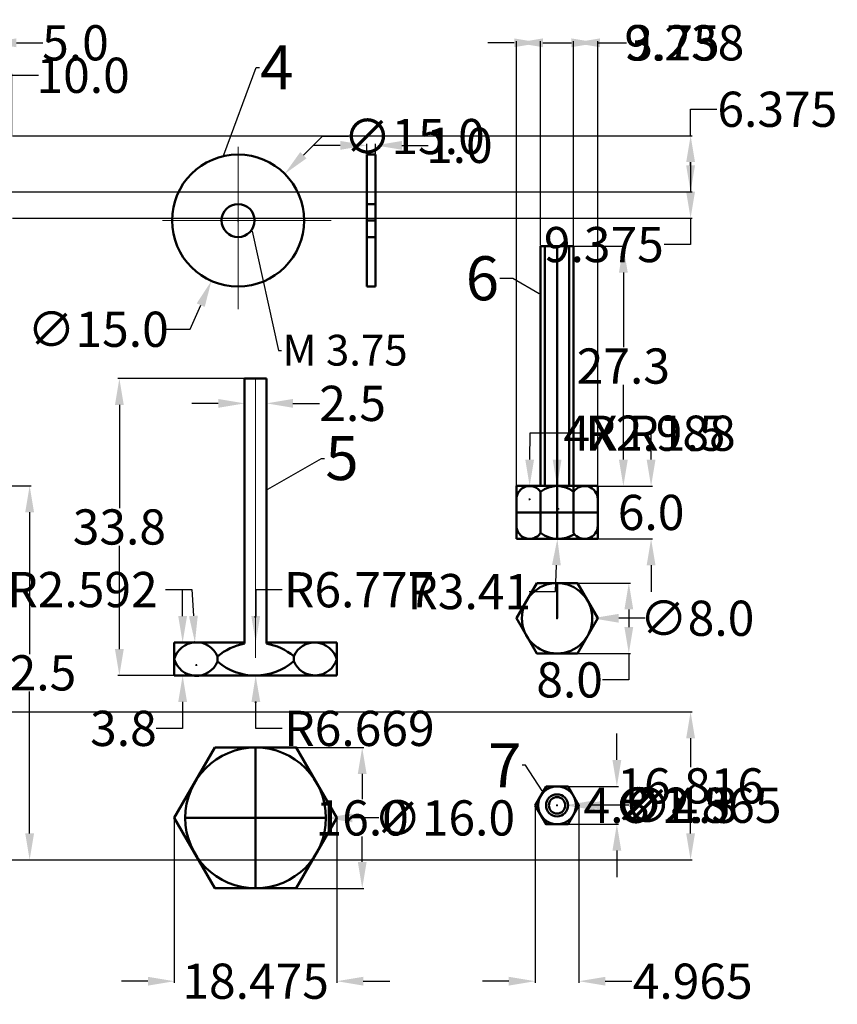
# Model space of a CAD drawing. Units: inches. Extents: x 0 to 231, y -13 to 111.
# Tile 3 of 3: x 138 to 231, y -13 to 98. Entities that reach past the tile are written whole.
import ezdxf
from ezdxf import colors
from ezdxf.entities.mleader import LeaderData, LeaderLine
from ezdxf.math import Vec2, Vec3

# ---------------------------------------------------------------- set-up
doc = ezdxf.new("R2010")
doc.units = ezdxf.units.IN
doc.header["$MEASUREMENT"] = 0
doc.linetypes.add('CENTER', pattern=[50.8, 31.75, -6.35, 6.35, -6.35])
for name, color, linetype, lineweight in [('M-CNTR', 1, 'CENTER', 18), ('M-DIMS', 2, 'Continuous', 25), ('M-OUTL', 7, 'Continuous', 50), ('M-TEXT', 3, 'Continuous', 25)]:
    doc.layers.add(name, color=color, linetype=linetype, lineweight=lineweight)
doc.styles.get("Standard").update_dxf_attribs({"font": 'arial.ttf'})
doc.dimstyles.get("Standard").update_dxf_attribs({"dimtxt": 4, "dimasz": 3, "dimexe": 0.18, "dimexo": 0.0625, "dimgap": 0.09, "dimtad": 0, "dimtih": 1, "dimtoh": 1, "dimdec": 1, "dimzin": 0, "dimdsep": 46, "dimtxsty": 'Standard', "dimcen": 0.09, "dimadec": 0, "dimazin": 0, "dimtfac": 1, "dimtdec": 1, "dimtofl": 0, "dimtmove": 0, "dimatfit": 3, "dimfxl": 1, "dimtolj": 1, "dimtzin": 0, "dimarcsym": 0})

# ---------------------------------------------------------------- blocks, each defined once
blk = doc.blocks.new('*D7')
at = {"layer": 'Defpoints', "color": 0, "transparency": 16777216}
for p in [(136.95, 92.07), (126.95, 85.21), (136.95, 85.21)]:
    blk.add_point(p, dxfattribs=at)
at = {"layer": 'M-DIMS', "color": 0, "lineweight": -2, "transparency": 16777216}
for p, q in [((126.95, 85.27), (126.95, 92.25)), ((129.95, 92.07), (133.95, 92.07)), ((136.95, 85.27), (136.95, 92.25)), ((136.95, 92.07), (139.95, 92.07))]:
    blk.add_line(p, q, dxfattribs=at)
at = {"layer": 'M-DIMS', "color": 0, "transparency": 16777216}
for points in [[(129.95, 92.57), (129.95, 91.57), (126.95, 92.07)], [(133.95, 92.57), (133.95, 91.57), (136.95, 92.07)]]:
    blk.add_solid(points, dxfattribs=at)
at = {"layer": 'M-DIMS', "color": 0, "transparency": 16777216, "insert": (145.04, 92.07), "char_height": 4, "attachment_point": 5}
blk.add_mtext('\\A1;10.0', dxfattribs=at)
blk = doc.blocks.new('*D17')
at = {"layer": 'Defpoints', "color": 0, "transparency": 16777216}
for p in [(120.95, 45.44), (120.95, 2.94), (138.96, 2.94)]:
    blk.add_point(p, dxfattribs=at)
at = {"layer": 'M-DIMS', "color": 0, "lineweight": -2, "transparency": 16777216}
for p, q in [((121.01, 45.44), (139.14, 45.44)), ((138.96, 42.44), (138.96, 26.33)), ((138.96, 5.94), (138.96, 22.06)), ((121.01, 2.94), (139.14, 2.94))]:
    blk.add_line(p, q, dxfattribs=at)
at = {"layer": 'M-DIMS', "color": 0, "transparency": 16777216}
for points in [[(138.46, 42.44), (139.46, 42.44), (138.96, 45.44)], [(138.46, 5.94), (139.46, 5.94), (138.96, 2.94)]]:
    blk.add_solid(points, dxfattribs=at)
at = {"layer": 'M-DIMS', "color": 0, "transparency": 16777216, "insert": (138.96, 24.19), "char_height": 4, "attachment_point": 5}
blk.add_mtext('\\A1;42.5', dxfattribs=at)
blk = doc.blocks.new('*D20')
at = {"layer": 'Defpoints', "color": 0, "transparency": 16777216}
for p in [(165.67, 82.43), (159.62, 68.71)]:
    blk.add_point(p, dxfattribs=at)
at = {"layer": 'M-DIMS', "color": 0, "lineweight": -2, "transparency": 16777216}
for p, q in [((162.56, 75.57), (162.74, 75.57)), ((162.65, 75.48), (162.65, 75.66)), ((157.2, 63.22), (158.41, 65.96)), ((154.2, 63.22), (157.2, 63.22))]:
    blk.add_line(p, q, dxfattribs=at)
at = {"layer": 'M-DIMS', "color": 0, "transparency": 16777216}
blk.add_solid([(157.95, 66.16), (158.86, 65.76), (159.62, 68.71)], dxfattribs=at)
at = {"layer": 'M-DIMS', "color": 0, "transparency": 16777216, "insert": (146.74, 63.22), "char_height": 4, "attachment_point": 5}
blk.add_mtext('\\A1;∅15.0', dxfattribs=at)
blk = doc.blocks.new('*D21')
at = {"layer": 'Defpoints', "color": 0, "transparency": 16777216}
for p in [(178.27, 84.11), (177.27, 83.07), (178.27, 83.07)]:
    blk.add_point(p, dxfattribs=at)
at = {"layer": 'M-DIMS', "color": 0, "lineweight": -2, "transparency": 16777216}
for p, q in [((174.27, 84.11), (171.27, 84.11)), ((177.27, 83.13), (177.27, 84.29)), ((178.27, 83.13), (178.27, 84.29)), ((181.27, 84.11), (184.27, 84.11))]:
    blk.add_line(p, q, dxfattribs=at)
at = {"layer": 'M-DIMS', "color": 0, "transparency": 16777216}
for points in [[(174.27, 84.61), (174.27, 83.61), (177.27, 84.11)], [(181.27, 84.61), (181.27, 83.61), (178.27, 84.11)]]:
    blk.add_solid(points, dxfattribs=at)
at = {"layer": 'M-DIMS', "color": 0, "transparency": 16777216, "insert": (187.8, 84.11), "char_height": 4, "attachment_point": 5}
blk.add_mtext('\\A1;1.0', dxfattribs=at)
blk = doc.blocks.new('*D22')
at = {"layer": 'Defpoints', "color": 0, "transparency": 16777216}
for p in [(164.64, 57.63), (149.16, 23.88), (164.59, 23.88)]:
    blk.add_point(p, dxfattribs=at)
at = {"layer": 'M-DIMS', "color": 0, "lineweight": -2, "transparency": 16777216}
for p, q in [((164.58, 57.63), (148.98, 57.63)), ((149.16, 54.63), (149.16, 42.89)), ((149.16, 26.88), (149.16, 38.62)), ((164.53, 23.88), (148.98, 23.88))]:
    blk.add_line(p, q, dxfattribs=at)
at = {"layer": 'M-DIMS', "color": 0, "transparency": 16777216}
for points in [[(148.66, 54.63), (149.66, 54.63), (149.16, 57.63)], [(148.66, 26.88), (149.66, 26.88), (149.16, 23.88)]]:
    blk.add_solid(points, dxfattribs=at)
at = {"layer": 'M-DIMS', "color": 0, "transparency": 16777216, "insert": (149.16, 40.76), "char_height": 4, "attachment_point": 5}
blk.add_mtext('\\A1;33.8', dxfattribs=at)
blk = doc.blocks.new('*D23')
at = {"layer": 'Defpoints', "color": 0, "transparency": 16777216}
for p in [(155.41, 27.63), (155.41, 23.88), (156.35, 23.88)]:
    blk.add_point(p, dxfattribs=at)
at = {"layer": 'M-DIMS', "color": 0, "lineweight": -2, "transparency": 16777216}
for p, q in [((156.35, 30.63), (156.35, 33.63)), ((155.47, 27.63), (156.53, 27.63)), ((155.47, 23.88), (156.53, 23.88)), ((156.35, 20.88), (156.35, 17.88)), ((156.35, 17.88), (153.35, 17.88))]:
    blk.add_line(p, q, dxfattribs=at)
at = {"layer": 'M-DIMS', "color": 0, "transparency": 16777216}
for points in [[(155.85, 30.63), (156.85, 30.63), (156.35, 27.63)], [(155.85, 20.88), (156.85, 20.88), (156.35, 23.88)]]:
    blk.add_solid(points, dxfattribs=at)
at = {"layer": 'M-DIMS', "color": 0, "transparency": 16777216, "insert": (149.62, 17.88), "char_height": 4, "attachment_point": 5}
blk.add_mtext('\\A1;3.8', dxfattribs=at)
blk = doc.blocks.new('*D24')
at = {"layer": 'Defpoints', "color": 0, "transparency": 16777216}
for p in [(164.64, 15.71), (164.64, -0.29), (176.76, -0.29)]:
    blk.add_point(p, dxfattribs=at)
at = {"layer": 'M-DIMS', "color": 0, "lineweight": -2, "transparency": 16777216}
for p, q in [((164.71, 15.71), (176.94, 15.71)), ((176.76, 12.71), (176.76, 9.84)), ((176.76, 2.71), (176.76, 5.58)), ((164.71, -0.29), (176.94, -0.29))]:
    blk.add_line(p, q, dxfattribs=at)
at = {"layer": 'M-DIMS', "color": 0, "transparency": 16777216}
for points in [[(176.26, 12.71), (177.26, 12.71), (176.76, 15.71)], [(176.26, 2.71), (177.26, 2.71), (176.76, -0.29)]]:
    blk.add_solid(points, dxfattribs=at)
at = {"layer": 'M-DIMS', "color": 0, "transparency": 16777216, "insert": (176.76, 7.71), "char_height": 4, "attachment_point": 5}
blk.add_mtext('\\A1;16.0', dxfattribs=at)
blk = doc.blocks.new('*D25')
at = {"layer": 'Defpoints', "color": 0, "transparency": 16777216}
for p in [(163.39, 53.99), (165.89, 54.8), (165.89, 54.36)]:
    blk.add_point(p, dxfattribs=at)
at = {"layer": 'M-DIMS', "color": 0, "lineweight": -2, "transparency": 16777216}
for p, q in [((163.39, 54.05), (163.39, 54.98)), ((165.89, 54.42), (165.89, 54.98)), ((160.39, 54.8), (157.39, 54.8)), ((168.89, 54.8), (171.89, 54.8))]:
    blk.add_line(p, q, dxfattribs=at)
at = {"layer": 'M-DIMS', "color": 0, "transparency": 16777216}
for points in [[(160.39, 55.3), (160.39, 54.3), (163.39, 54.8)], [(168.89, 55.3), (168.89, 54.3), (165.89, 54.8)]]:
    blk.add_solid(points, dxfattribs=at)
at = {"layer": 'M-DIMS', "color": 0, "transparency": 16777216, "insert": (175.67, 54.8), "char_height": 4, "attachment_point": 5}
blk.add_mtext('\\A1;2.5', dxfattribs=at)
blk = doc.blocks.new('*D26')
at = {"layer": 'Defpoints', "color": 0, "transparency": 16777216}
for p in [(203.53, 45.41), (203.53, 39.41), (209.59, 39.41)]:
    blk.add_point(p, dxfattribs=at)
at = {"layer": 'M-DIMS', "color": 0, "lineweight": -2, "transparency": 16777216}
for p, q in [((209.59, 48.41), (209.59, 51.41)), ((203.59, 45.41), (209.77, 45.41)), ((203.59, 39.41), (209.77, 39.41)), ((209.59, 36.41), (209.59, 33.41))]:
    blk.add_line(p, q, dxfattribs=at)
at = {"layer": 'M-DIMS', "color": 0, "transparency": 16777216}
for points in [[(209.09, 48.41), (210.09, 48.41), (209.59, 45.41)], [(209.09, 36.41), (210.09, 36.41), (209.59, 39.41)]]:
    blk.add_solid(points, dxfattribs=at)
at = {"layer": 'M-DIMS', "color": 0, "transparency": 16777216, "insert": (209.59, 42.41), "char_height": 4, "attachment_point": 5}
blk.add_mtext('\\A1;6.0', dxfattribs=at)
blk = doc.blocks.new('*D27')
at = {"layer": 'Defpoints', "color": 0, "transparency": 16777216}
for p in [(198.91, 72.66), (198.91, 45.41), (206.44, 45.41)]:
    blk.add_point(p, dxfattribs=at)
at = {"layer": 'M-DIMS', "color": 0, "lineweight": -2, "transparency": 16777216}
for p, q in [((198.97, 72.66), (206.62, 72.66)), ((206.44, 69.66), (206.44, 61.17)), ((206.44, 48.41), (206.44, 56.91)), ((198.97, 45.41), (206.62, 45.41))]:
    blk.add_line(p, q, dxfattribs=at)
at = {"layer": 'M-DIMS', "color": 0, "transparency": 16777216}
for points in [[(205.94, 69.66), (206.94, 69.66), (206.44, 72.66)], [(205.94, 48.41), (206.94, 48.41), (206.44, 45.41)]]:
    blk.add_solid(points, dxfattribs=at)
at = {"layer": 'M-DIMS', "color": 0, "transparency": 16777216, "insert": (206.44, 59.04), "char_height": 4, "attachment_point": 5}
blk.add_mtext('\\A1;27.3', dxfattribs=at)
blk = doc.blocks.new('*D28')
at = {"layer": 'Defpoints', "color": 0, "transparency": 16777216}
for p in [(198.91, 34.39), (198.91, 26.39), (207.06, 26.39)]:
    blk.add_point(p, dxfattribs=at)
at = {"layer": 'M-DIMS', "color": 0, "lineweight": -2, "transparency": 16777216}
for p, q in [((198.97, 34.39), (207.24, 34.39)), ((207.06, 31.39), (207.06, 29.39)), ((198.97, 26.39), (207.24, 26.39)), ((207.06, 26.39), (207.06, 23.39)), ((207.06, 23.39), (204.06, 23.39))]:
    blk.add_line(p, q, dxfattribs=at)
at = {"layer": 'M-DIMS', "color": 0, "transparency": 16777216}
for points in [[(206.56, 31.39), (207.56, 31.39), (207.06, 34.39)], [(206.56, 29.39), (207.56, 29.39), (207.06, 26.39)]]:
    blk.add_solid(points, dxfattribs=at)
at = {"layer": 'M-DIMS', "color": 0, "transparency": 16777216, "insert": (200.33, 23.39), "char_height": 4, "attachment_point": 5}
blk.add_mtext('\\A1;8.0', dxfattribs=at)
blk = doc.blocks.new('*D29')
at = {"layer": 'Defpoints', "color": 0, "transparency": 16777216}
for p in [(198.91, 11.29), (198.91, 6.99), (205.7, 6.99)]:
    blk.add_point(p, dxfattribs=at)
at = {"layer": 'M-DIMS', "color": 0, "lineweight": -2, "transparency": 16777216}
for p, q in [((205.7, 14.29), (205.7, 17.29)), ((198.97, 11.29), (205.88, 11.29)), ((198.97, 6.99), (205.88, 6.99)), ((205.7, 3.99), (205.7, 0.99))]:
    blk.add_line(p, q, dxfattribs=at)
at = {"layer": 'M-DIMS', "color": 0, "transparency": 16777216}
for points in [[(205.2, 14.29), (206.2, 14.29), (205.7, 11.29)], [(205.2, 3.99), (206.2, 3.99), (205.7, 6.99)]]:
    blk.add_solid(points, dxfattribs=at)
at = {"layer": 'M-DIMS', "color": 0, "transparency": 16777216, "insert": (205.7, 9.14), "char_height": 4, "attachment_point": 5}
blk.add_mtext('\\A1;4.3', dxfattribs=at)
blk = doc.blocks.new('*D34')
at = {"layer": 'Defpoints', "color": 0, "transparency": 16777216}
for p in [(134.45, 95.76), (129.45, 85.21), (134.45, 85.21)]:
    blk.add_point(p, dxfattribs=at)
at = {"layer": 'M-DIMS', "color": 0, "lineweight": -2, "transparency": 16777216}
for p, q in [((126.45, 95.76), (123.45, 95.76)), ((129.45, 85.27), (129.45, 95.94)), ((134.45, 85.27), (134.45, 95.94)), ((137.45, 95.76), (140.45, 95.76))]:
    blk.add_line(p, q, dxfattribs=at)
at = {"layer": 'M-DIMS', "color": 0, "transparency": 16777216}
for points in [[(126.45, 96.26), (126.45, 95.26), (129.45, 95.76)], [(137.45, 96.26), (137.45, 95.26), (134.45, 95.76)]]:
    blk.add_solid(points, dxfattribs=at)
at = {"layer": 'M-DIMS', "color": 0, "transparency": 16777216, "insert": (144.17, 95.76), "char_height": 4, "attachment_point": 5}
blk.add_mtext('\\A1;5.0', dxfattribs=at)
blk = doc.blocks.new('*D35')
at = {"layer": 'Defpoints', "color": 0, "transparency": 16777216}
for p in [(136.95, 85.21), (214.08, 85.21), (131.95, 78.84)]:
    blk.add_point(p, dxfattribs=at)
at = {"layer": 'M-DIMS', "color": 0, "lineweight": -2, "transparency": 16777216}
for p, q in [((214.08, 85.21), (214.08, 88.21)), ((214.08, 88.21), (217.08, 88.21)), ((137.01, 85.21), (214.26, 85.21)), ((214.08, 81.84), (214.08, 82.21)), ((132.01, 78.84), (214.26, 78.84))]:
    blk.add_line(p, q, dxfattribs=at)
at = {"layer": 'M-DIMS', "color": 0, "transparency": 16777216}
for points in [[(213.58, 82.21), (214.58, 82.21), (214.08, 85.21)], [(213.58, 81.84), (214.58, 81.84), (214.08, 78.84)]]:
    blk.add_solid(points, dxfattribs=at)
at = {"layer": 'M-DIMS', "color": 0, "transparency": 16777216, "insert": (223.94, 88.21), "char_height": 4, "attachment_point": 5}
blk.add_mtext('\\A1;6.375', dxfattribs=at)
blk = doc.blocks.new('*D36')
at = {"layer": 'Defpoints', "color": 0, "transparency": 16777216}
for p in [(136.95, 85.21), (136.95, 75.84), (214.08, 75.84)]:
    blk.add_point(p, dxfattribs=at)
at = {"layer": 'M-DIMS', "color": 0, "lineweight": -2, "transparency": 16777216}
for p, q in [((137.01, 85.21), (214.26, 85.21)), ((214.08, 82.21), (214.08, 78.84)), ((137.01, 75.84), (214.26, 75.84)), ((214.08, 75.84), (214.08, 72.84)), ((214.08, 72.84), (211.08, 72.84))]:
    blk.add_line(p, q, dxfattribs=at)
at = {"layer": 'M-DIMS', "color": 0, "transparency": 16777216}
for points in [[(213.58, 82.21), (214.58, 82.21), (214.08, 85.21)], [(213.58, 78.84), (214.58, 78.84), (214.08, 75.84)]]:
    blk.add_solid(points, dxfattribs=at)
at = {"layer": 'M-DIMS', "color": 0, "transparency": 16777216, "insert": (204.22, 72.84), "char_height": 4, "attachment_point": 5}
blk.add_mtext('\\A1;9.375', dxfattribs=at)
blk = doc.blocks.new('*D45')
at = {"layer": 'Defpoints', "color": 0, "transparency": 16777216}
for p in [(119.7, 19.76), (120.95, 2.94), (214.08, 2.94)]:
    blk.add_point(p, dxfattribs=at)
at = {"layer": 'M-DIMS', "color": 0, "lineweight": -2, "transparency": 16777216}
for p, q in [((119.76, 19.76), (214.26, 19.76)), ((214.08, 16.76), (214.08, 13.48)), ((214.08, 5.94), (214.08, 9.22)), ((121.01, 2.94), (214.26, 2.94))]:
    blk.add_line(p, q, dxfattribs=at)
at = {"layer": 'M-DIMS', "color": 0, "transparency": 16777216}
for points in [[(213.58, 16.76), (214.58, 16.76), (214.08, 19.76)], [(213.58, 5.94), (214.58, 5.94), (214.08, 2.94)]]:
    blk.add_solid(points, dxfattribs=at)
at = {"layer": 'M-DIMS', "color": 0, "transparency": 16777216, "insert": (214.08, 11.35), "char_height": 4, "attachment_point": 5}
blk.add_mtext('\\A1;16.816', dxfattribs=at)
blk = doc.blocks.new('*D47')
at = {"layer": 'Defpoints', "color": 0, "transparency": 16777216}
for p in [(155.405372, 7.711161), (173.88058, 7.711161), (173.88058, -10.838839)]:
    blk.add_point(p, dxfattribs=at)
at = {"layer": 'M-DIMS', "color": 0, "lineweight": -2, "transparency": 16777216}
for p, q in [((155.405372, 7.648661), (155.405372, -11.018839)), ((173.88058, 7.648661), (173.88058, -11.018839)), ((152.405372, -10.838839), (149.405372, -10.838839)), ((176.88058, -10.838839), (179.88058, -10.838839))]:
    blk.add_line(p, q, dxfattribs=at)
at = {"layer": 'M-DIMS', "color": 0, "transparency": 16777216}
for points in [[(152.405372, -10.338839), (152.405372, -11.338839), (155.405372, -10.838839)], [(176.88058, -10.338839), (176.88058, -11.338839), (173.88058, -10.838839)]]:
    blk.add_solid(points, dxfattribs=at)
at = {"layer": 'M-DIMS', "color": 0, "transparency": 16777216, "insert": (164.642976, -10.838839), "char_height": 4, "attachment_point": 5}
blk.add_mtext('\\A1;18.475', dxfattribs=at)
blk = doc.blocks.new('*D48')
at = {"layer": 'Defpoints', "color": 0, "transparency": 16777216}
for p in [(203.53, 95.76), (194.29, 45.41), (203.53, 45.41)]:
    blk.add_point(p, dxfattribs=at)
at = {"layer": 'M-DIMS', "color": 0, "lineweight": -2, "transparency": 16777216}
for p, q in [((194.29, 45.48), (194.29, 95.94)), ((197.29, 95.76), (200.53, 95.76)), ((203.53, 45.48), (203.53, 95.94)), ((203.53, 95.76), (206.53, 95.76))]:
    blk.add_line(p, q, dxfattribs=at)
at = {"layer": 'M-DIMS', "color": 0, "transparency": 16777216}
for points in [[(197.29, 96.26), (197.29, 95.26), (194.29, 95.76)], [(200.53, 96.26), (200.53, 95.26), (203.53, 95.76)]]:
    blk.add_solid(points, dxfattribs=at)
at = {"layer": 'M-DIMS', "color": 0, "transparency": 16777216, "insert": (213.37, 95.76), "char_height": 4, "attachment_point": 5}
blk.add_mtext('\\A1;9.238', dxfattribs=at)
blk = doc.blocks.new('*D49')
at = {"layer": 'Defpoints', "color": 0, "transparency": 16777216}
for p in [(200.78, 95.76), (197.03, 72.66), (200.78, 72.66)]:
    blk.add_point(p, dxfattribs=at)
at = {"layer": 'M-DIMS', "color": 0, "lineweight": -2, "transparency": 16777216}
for p, q in [((194.03, 95.76), (191.03, 95.76)), ((197.03, 72.73), (197.03, 95.94)), ((200.78, 72.73), (200.78, 95.94)), ((203.78, 95.76), (206.78, 95.76))]:
    blk.add_line(p, q, dxfattribs=at)
at = {"layer": 'M-DIMS', "color": 0, "transparency": 16777216}
for points in [[(194.03, 96.26), (194.03, 95.26), (197.03, 95.76)], [(203.78, 96.26), (203.78, 95.26), (200.78, 95.76)]]:
    blk.add_solid(points, dxfattribs=at)
at = {"layer": 'M-DIMS', "color": 0, "transparency": 16777216, "insert": (212.08, 95.76), "char_height": 4, "attachment_point": 5}
blk.add_mtext('\\A1;3.75', dxfattribs=at)
blk = doc.blocks.new('*D50')
at = {"layer": 'Defpoints', "color": 0, "transparency": 16777216}
for p in [(196.42, 9.14), (201.39, 9.14), (201.39, -10.84)]:
    blk.add_point(p, dxfattribs=at)
at = {"layer": 'M-DIMS', "color": 0, "lineweight": -2, "transparency": 16777216}
for p, q in [((196.42, 9.08), (196.42, -11.02)), ((201.39, 9.08), (201.39, -11.02)), ((193.42, -10.84), (190.42, -10.84)), ((204.39, -10.84), (207.39, -10.84))]:
    blk.add_line(p, q, dxfattribs=at)
at = {"layer": 'M-DIMS', "color": 0, "transparency": 16777216}
for points in [[(193.42, -10.34), (193.42, -11.34), (196.42, -10.84)], [(204.39, -10.34), (204.39, -11.34), (201.39, -10.84)]]:
    blk.add_solid(points, dxfattribs=at)
at = {"layer": 'M-DIMS', "color": 0, "transparency": 16777216, "insert": (214.32, -10.84), "char_height": 4, "attachment_point": 5}
blk.add_mtext('\\A1;4.965', dxfattribs=at)
blk = doc.blocks.new('*D53')
at = {"layer": 'Defpoints', "color": 0, "transparency": 16777216}
for p in [(167.95, 80.87), (157.34, 70.27)]:
    blk.add_point(p, dxfattribs=at)
at = {"layer": 'M-DIMS', "color": 0, "lineweight": -2, "transparency": 16777216}
for p, q in [((172.19, 85.11), (170.07, 82.99)), ((175.19, 85.11), (172.19, 85.11)), ((162.56, 75.57), (162.74, 75.57)), ((162.65, 75.48), (162.65, 75.66))]:
    blk.add_line(p, q, dxfattribs=at)
at = {"layer": 'M-DIMS', "color": 0, "transparency": 16777216}
blk.add_solid([(169.72, 83.35), (170.43, 82.64), (167.95, 80.87)], dxfattribs=at)
at = {"layer": 'M-DIMS', "color": 0, "transparency": 16777216, "insert": (182.65, 85.11), "char_height": 4, "attachment_point": 5}
blk.add_mtext('\\A1;∅15.0', dxfattribs=at)
blk = doc.blocks.new('*D55')
at = {"layer": 'Defpoints', "color": 0, "transparency": 16777216}
for p in [(156.64, 7.71), (172.64, 7.71)]:
    blk.add_point(p, dxfattribs=at)
at = {"layer": 'M-DIMS', "color": 0, "lineweight": -2, "transparency": 16777216}
for p, q in [((164.55, 7.71), (164.73, 7.71)), ((164.64, 7.62), (164.64, 7.8)), ((178.64, 7.71), (175.64, 7.71))]:
    blk.add_line(p, q, dxfattribs=at)
at = {"layer": 'M-DIMS', "color": 0, "transparency": 16777216}
blk.add_solid([(175.64, 8.21), (175.64, 7.21), (172.64, 7.71)], dxfattribs=at)
at = {"layer": 'M-DIMS', "color": 0, "transparency": 16777216, "insert": (186.1, 7.71), "char_height": 4, "attachment_point": 5}
blk.add_mtext('\\A1;∅16.0', dxfattribs=at)
blk = doc.blocks.new('*D56')
at = {"layer": 'Defpoints', "color": 0, "transparency": 16777216}
for p in [(164.66, 27.63), (164.66, 20.86)]:
    blk.add_point(p, dxfattribs=at)
at = {"layer": 'M-DIMS', "color": 0, "lineweight": -2, "transparency": 16777216}
for p, q in [((167.66, 33.63), (164.66, 33.63)), ((164.66, 33.63), (164.66, 30.63)), ((164.57, 20.86), (164.75, 20.86)), ((164.66, 20.77), (164.66, 20.95))]:
    blk.add_line(p, q, dxfattribs=at)
at = {"layer": 'M-DIMS', "color": 0, "transparency": 16777216}
blk.add_solid([(164.16, 30.63), (165.16, 30.63), (164.66, 27.63)], dxfattribs=at)
at = {"layer": 'M-DIMS', "color": 0, "transparency": 16777216, "insert": (176.41, 33.63), "char_height": 4, "attachment_point": 5}
blk.add_mtext('\\A1;R6.777', dxfattribs=at)
blk = doc.blocks.new('*D57')
at = {"layer": 'Defpoints', "color": 0, "transparency": 16777216}
for p in [(164.62, 30.55), (164.65, 23.88)]:
    blk.add_point(p, dxfattribs=at)
at = {"layer": 'M-DIMS', "color": 0, "lineweight": -2, "transparency": 16777216}
for p, q in [((164.53, 30.55), (164.71, 30.55)), ((164.62, 30.46), (164.62, 30.64)), ((164.68, 17.88), (164.67, 20.88)), ((167.68, 17.88), (164.68, 17.88))]:
    blk.add_line(p, q, dxfattribs=at)
at = {"layer": 'M-DIMS', "color": 0, "transparency": 16777216}
blk.add_solid([(165.17, 20.89), (164.17, 20.88), (164.65, 23.88)], dxfattribs=at)
at = {"layer": 'M-DIMS', "color": 0, "transparency": 16777216, "insert": (176.44, 17.88), "char_height": 4, "attachment_point": 5}
blk.add_mtext('\\A1;R6.669', dxfattribs=at)
blk = doc.blocks.new('*D58')
at = {"layer": 'Defpoints', "color": 0, "transparency": 16777216}
for p in [(157.75, 27.66), (157.91, 25.07)]:
    blk.add_point(p, dxfattribs=at)
at = {"layer": 'M-DIMS', "color": 0, "lineweight": -2, "transparency": 16777216}
for p, q in [((154.39, 33.65), (157.39, 33.65)), ((157.39, 33.65), (157.57, 30.65)), ((157.82, 25.07), (158, 25.07)), ((157.91, 24.98), (157.91, 25.16))]:
    blk.add_line(p, q, dxfattribs=at)
at = {"layer": 'M-DIMS', "color": 0, "transparency": 16777216}
blk.add_solid([(158.07, 30.68), (157.07, 30.62), (157.75, 27.66)], dxfattribs=at)
at = {"layer": 'M-DIMS', "color": 0, "transparency": 16777216, "insert": (141.28, 33.65), "char_height": 4, "attachment_point": 5}
blk.add_mtext('\\A1;4X R2.592', dxfattribs=at)
blk = doc.blocks.new('*D59')
at = {"layer": 'Defpoints', "color": 0, "transparency": 16777216}
for p in [(195.79, 45.41), (195.79, 43.91)]:
    blk.add_point(p, dxfattribs=at)
at = {"layer": 'M-DIMS', "color": 0, "lineweight": -2, "transparency": 16777216}
for p, q in [((195.8, 51.41), (195.79, 48.41)), ((198.8, 51.41), (195.8, 51.41)), ((195.7, 43.91), (195.88, 43.91)), ((195.79, 43.82), (195.79, 44))]:
    blk.add_line(p, q, dxfattribs=at)
at = {"layer": 'M-DIMS', "color": 0, "transparency": 16777216}
blk.add_solid([(195.29, 48.42), (196.29, 48.41), (195.79, 45.41)], dxfattribs=at)
at = {"layer": 'M-DIMS', "color": 0, "transparency": 16777216, "insert": (208.84, 51.41), "char_height": 4, "attachment_point": 5}
blk.add_mtext('\\A1;4X R1.5', dxfattribs=at)
blk = doc.blocks.new('*D60')
at = {"layer": 'Defpoints', "color": 0, "transparency": 16777216}
for p in [(199.05, 42.82), (198.94, 39.41)]:
    blk.add_point(p, dxfattribs=at)
at = {"layer": 'M-DIMS', "color": 0, "lineweight": -2, "transparency": 16777216}
for p, q in [((198.96, 42.82), (199.14, 42.82)), ((199.05, 42.73), (199.05, 42.91)), ((198.73, 33.42), (198.83, 36.42)), ((195.73, 33.42), (198.73, 33.42))]:
    blk.add_line(p, q, dxfattribs=at)
at = {"layer": 'M-DIMS', "color": 0, "transparency": 16777216}
blk.add_solid([(198.33, 36.43), (199.33, 36.4), (198.94, 39.41)], dxfattribs=at)
at = {"layer": 'M-DIMS', "color": 0, "transparency": 16777216, "insert": (188.92, 33.42), "char_height": 4, "attachment_point": 5}
blk.add_mtext('\\A1;R3.41', dxfattribs=at)
blk = doc.blocks.new('*D61')
at = {"layer": 'Defpoints', "color": 0, "transparency": 16777216}
for p in [(198.91, 45.41), (198.91, 42.43)]:
    blk.add_point(p, dxfattribs=at)
at = {"layer": 'M-DIMS', "color": 0, "lineweight": -2, "transparency": 16777216}
for p, q in [((201.91, 51.41), (198.91, 51.41)), ((198.91, 51.41), (198.91, 48.41)), ((198.91, 42.34), (198.91, 42.52)), ((198.82, 42.43), (199, 42.43))]:
    blk.add_line(p, q, dxfattribs=at)
at = {"layer": 'M-DIMS', "color": 0, "transparency": 16777216}
blk.add_solid([(198.41, 48.41), (199.41, 48.41), (198.91, 45.41)], dxfattribs=at)
at = {"layer": 'M-DIMS', "color": 0, "transparency": 16777216, "insert": (210.66, 51.41), "char_height": 4, "attachment_point": 5}
blk.add_mtext('\\A1;R2.988', dxfattribs=at)
blk = doc.blocks.new('*D62')
at = {"layer": 'Defpoints', "color": 0, "transparency": 16777216}
for p in [(194.91, 30.39), (202.91, 30.39)]:
    blk.add_point(p, dxfattribs=at)
at = {"layer": 'M-DIMS', "color": 0, "lineweight": -2, "transparency": 16777216}
for p, q in [((198.82, 30.39), (199, 30.39)), ((198.91, 30.3), (198.91, 30.48)), ((208.91, 30.39), (205.91, 30.39))]:
    blk.add_line(p, q, dxfattribs=at)
at = {"layer": 'M-DIMS', "color": 0, "transparency": 16777216}
blk.add_solid([(205.91, 30.89), (205.91, 29.89), (202.91, 30.39)], dxfattribs=at)
at = {"layer": 'M-DIMS', "color": 0, "transparency": 16777216, "insert": (214.81, 30.39), "char_height": 4, "attachment_point": 5}
blk.add_mtext('\\A1;∅8.0', dxfattribs=at)
blk = doc.blocks.new('*D63')
at = {"layer": 'Defpoints', "color": 0, "transparency": 16777216}
for p in [(196.76, 9.14), (201.06, 9.14)]:
    blk.add_point(p, dxfattribs=at)
at = {"layer": 'M-DIMS', "color": 0, "lineweight": -2, "transparency": 16777216}
for p, q in [((198.82, 9.14), (199, 9.14)), ((198.91, 9.05), (198.91, 9.23)), ((207.06, 9.14), (204.06, 9.14))]:
    blk.add_line(p, q, dxfattribs=at)
at = {"layer": 'M-DIMS', "color": 0, "transparency": 16777216}
blk.add_solid([(204.06, 9.64), (204.06, 8.64), (201.06, 9.14)], dxfattribs=at)
at = {"layer": 'M-DIMS', "color": 0, "transparency": 16777216, "insert": (212.96, 9.14), "char_height": 4, "attachment_point": 5}
blk.add_mtext('\\A1;∅4.3', dxfattribs=at)
blk = doc.blocks.new('*D64')
at = {"layer": 'Defpoints', "color": 0, "transparency": 16777216}
for p in [(197.66, 9.14), (200.16, 9.14)]:
    blk.add_point(p, dxfattribs=at)
at = {"layer": 'M-DIMS', "color": 0, "lineweight": -2, "transparency": 16777216}
for p, q in [((198.82, 9.14), (199, 9.14)), ((198.91, 9.05), (198.91, 9.23)), ((206.16, 9.15), (203.16, 9.14))]:
    blk.add_line(p, q, dxfattribs=at)
at = {"layer": 'M-DIMS', "color": 0, "transparency": 16777216}
blk.add_solid([(203.16, 9.64), (203.16, 8.64), (200.16, 9.14)], dxfattribs=at)
at = {"layer": 'M-DIMS', "color": 0, "transparency": 16777216, "insert": (212.08, 9.15), "char_height": 4, "attachment_point": 5}
blk.add_mtext('\\A1;∅2.5', dxfattribs=at)
blk = doc.blocks.new('*D65')
at = {"layer": 'Defpoints', "color": 0, "transparency": 16777216}
for p in [(197.97, 9.14), (199.84, 9.14)]:
    blk.add_point(p, dxfattribs=at)
at = {"layer": 'M-DIMS', "color": 0, "lineweight": -2, "transparency": 16777216}
for p, q in [((198.82, 9.14), (199, 9.14)), ((198.91, 9.05), (198.91, 9.23)), ((205.84, 9.15), (202.84, 9.15))]:
    blk.add_line(p, q, dxfattribs=at)
at = {"layer": 'M-DIMS', "color": 0, "transparency": 16777216}
blk.add_solid([(202.84, 9.65), (202.84, 8.65), (199.84, 9.14)], dxfattribs=at)
at = {"layer": 'M-DIMS', "color": 0, "transparency": 16777216, "insert": (214.87, 9.15), "char_height": 4, "attachment_point": 5}
blk.add_mtext('\\A1;∅1.865', dxfattribs=at)

msp = doc.modelspace()

# ---------------------------------------------------------------- linework, layer by layer
at = {"layer": 'M-CNTR'}
for p, q in [((162.6462, 65.5196), (162.6462, 83.9575)), ((154.0559, 75.5682), (173.2454, 75.5682)), ((164.643, 57.6328), (164.643, 20.2824))]:
    msp.add_line(p, q, dxfattribs=at)
at = {"layer": 'M-OUTL'}
for p, q in [((177.2674, 83.0682), (178.2674, 83.0682)), ((177.2674, 83.0682), (177.2674, 68.0682)), ((178.2674, 83.0682), (178.2674, 68.0682)), ((177.2674, 77.4432), (178.2674, 77.4432)), ((177.2674, 75.5682), (178.2674, 75.5682)), ((177.2674, 73.6932), (178.2674, 73.6932)), ((197.0319, 72.6646), (200.7819, 72.6646)), ((197.0319, 45.4146), (197.0319, 72.6646)), ((197.5319, 45.4146), (197.5319, 72.6646)), ((198.9069, 39.4146), (198.9069, 72.6646)), ((200.2819, 45.4146), (200.2819, 72.6646)), ((200.7819, 40.0761), (200.7819, 72.6646)), ((177.2674, 68.0682), (178.2674, 68.0682)), ((163.393, 57.6328), (165.893, 57.6328)), ((163.393, 57.6328), (163.393, 27.5141)), ((165.893, 57.6328), (165.893, 27.5189)), ((194.2881, 39.4146), (194.2881, 45.4146)), ((194.2881, 45.4146), (203.5257, 45.4146)), ((197.0319, 40.0761), (197.0319, 44.753)), ((203.5257, 39.4146), (203.5257, 45.4146)), ((194.2881, 42.4146), (203.5257, 42.4146)), ((194.2881, 39.4146), (203.5257, 39.4146)), ((198.9069, 30.3883), (198.9069, 34.3883)), ((155.4054, 23.8828), (155.4054, 27.6328)), ((155.4054, 27.6328), (163.393, 27.6328)), ((164.643, 27.6328), (164.6687, 27.6328)), ((165.893, 27.6328), (173.8806, 27.6328)), ((173.8806, 23.8828), (173.8806, 27.6328)), ((160.3054, 25.4635), (160.3054, 26.0521)), ((168.9806, 25.5088), (168.9806, 26.0735)), ((155.4054, 23.8828), (173.8806, 23.8828)), ((163.393, 23.9959), (163.393, 23.8828)), ((165.893, 24.006), (165.893, 23.8828)), ((164.643, 15.7112), (164.643, -0.2888)), ((156.643, 7.7112), (172.643, 7.7112))]:
    msp.add_line(p, q, dxfattribs=at)
for points in [[(196.5975, 34.3883), (194.2881, 30.3883), (196.5975, 26.3883), (201.2163, 26.3883), (203.5257, 30.3883), (201.2163, 34.3883)], [(160.0242, 15.7112), (155.4054, 7.7112), (160.0242, -0.2888), (169.2618, -0.2888), (173.8806, 7.7112), (169.2618, 15.7112)], [(197.6656, 11.288), (196.4243, 9.138), (197.6656, 6.988), (200.1482, 6.988), (201.3895, 9.138), (200.1482, 11.288)]]:
    msp.add_lwpolyline(points, close=True, dxfattribs=at)
for centre, radius in [((162.6462, 75.5682), 7.5), ((162.6462, 75.5682), 1.875), ((198.9069, 30.3883), 4), ((164.643, 7.7112), 8), ((198.9069, 9.138), 2.15), ((198.9069, 9.138), 1.25), ((198.9069, 9.138), 0.9325)]:
    msp.add_circle(centre, radius, dxfattribs=at)
for centre, radius, start, end in [((195.7881, 43.9146), 1.5, 33.983207, 180), ((198.9069, 42.4268), 2.9878, 51.130231, 128.869769), ((202.0257, 43.9146), 1.5, 0, 146.016793), ((195.7881, 40.9146), 1.5, 180, 326.016793), ((202.0257, 40.9146), 1.5, 213.983207, 0), ((199.0535, 42.8179), 3.4065, 233.597055, 302.466824), ((157.9054, 25.0724), 2.5922, 22.204863, 164.669131), ((164.6559, 20.8557), 6.7771, 100.739567, 129.936687), ((164.6559, 20.8557), 6.7771, 89.891154, 90.108846), ((164.6559, 20.8557), 6.7771, 50.34664, 79.481924), ((171.3581, 25.0405), 2.5922, 15.330869, 156.516195), ((157.9054, 26.4432), 2.5922, 195.330869, 337.795137), ((171.3806, 26.4885), 2.5922, 202.204863, 342.891494), ((164.6165, 30.5519), 6.6691, 229.726974, 310.87202)]:
    msp.add_arc(centre, radius, start, end, dxfattribs=at)

# ---------------------------------------------------------------- dimensions: what is measured, and where the dimension line sits
at = {"layer": 'M-DIMS'}
for base, p1, p2, override, picture, middle in [((134.4483, 95.7603), (129.4483, 85.2103), (134.4483, 85.2103), {"dimdec": 1, "dimlfac": 1, "dimrnd": 0, "dimzin": 0, "dimdsep": 46, "dimlunit": 2}, '*D34', (144.1727, 95.7603)), ((200.7819, 95.7603), (197.0319, 72.6646), (200.7819, 72.6646), {"dimdec": 2, "dimlfac": 1, "dimrnd": 0, "dimzin": 0, "dimdsep": 46, "dimlunit": 2}, '*D49', (212.0806, 95.7603)), ((203.5257, 95.7603), (194.2881, 45.4146), (203.5257, 45.4146), {"dimdec": 3, "dimlfac": 1, "dimrnd": 0, "dimzin": 0, "dimdsep": 46, "dimlunit": 2}, '*D48', (213.3687, 95.7603)), ((136.9483, 92.0651), (126.9483, 85.2103), (136.9483, 85.2103), {"dimclrd": 0, "dimclre": 0, "dimclrt": 0}, '*D7', (145.0383, 92.0651)), ((178.2674, 84.1081), (177.2674, 83.0682), (178.2674, 83.0682), {"dimclrd": 0, "dimclre": 0, "dimclrt": 0}, '*D21', (187.8035, 84.1081)), ((165.893, 54.8023), (163.393, 53.9904), (165.893, 54.3595), {"dimclrd": 0, "dimclre": 0, "dimclrt": 0}, '*D25', (175.6733, 54.8023)), ((201.3895, -10.8388), (196.4243, 9.138), (201.3895, 9.138), {"dimdec": 3, "dimlfac": 1, "dimrnd": 0, "dimzin": 0, "dimdsep": 46, "dimlunit": 2}, '*D50', (214.3239, -10.8388)), ((173.8806, -10.8388), (155.4054, 7.7112), (173.8806, 7.7112), {"dimdec": 3, "dimlfac": 1, "dimrnd": 0, "dimzin": 0, "dimdsep": 46, "dimlunit": 2}, '*D47', (164.643, -10.8388))]:
    dim = msp.add_linear_dim(base=base, p1=p1, p2=p2, dimstyle='Standard', override=override, dxfattribs=at)
    dim.commit()
    dim.dimension.update_dxf_attribs({"geometry": picture, "text_midpoint": middle})
for base, p1, p2, override, picture, middle in [((214.0757, 85.2103), (131.9483, 78.8353), (136.9483, 85.2103), {"dimdec": 3, "dimlfac": 1, "dimrnd": 0, "dimzin": 0, "dimdsep": 46, "dimlunit": 2}, '*D35', (223.9406, 88.2103)), ((214.0757, 75.8353), (136.9483, 85.2103), (136.9483, 75.8353), {"dimdec": 3, "dimlfac": 1, "dimrnd": 0, "dimzin": 0, "dimdsep": 46, "dimlunit": 2}, '*D36', (204.2217, 72.8353)), ((206.4415005475, 45.4145561365), (198.9068568321, 72.6645561365), (198.9068568321, 45.4145561365), {"dimclrd": 0, "dimclre": 0, "dimclrt": 0}, '*D27', (206.4415005475, 59.0395561365)), ((149.1648608381, 23.8827857643), (164.6429760605, 57.6327857643), (164.59001679, 23.8827857643), {"dimclrd": 0, "dimclre": 0, "dimclrt": 0}, '*D22', (149.1648608381, 40.7577857643)), ((209.5925, 39.4146), (203.5257, 45.4146), (203.5257, 39.4146), {"dimclrd": 0, "dimclre": 0, "dimclrt": 0}, '*D26', (209.5925, 42.4146)), ((138.9616, 2.9428), (120.9464, 45.4428), (120.9464, 2.9428), {"dimclrd": 0, "dimclre": 0, "dimclrt": 0}, '*D17', (138.9616, 24.1928)), ((156.3523328769, 23.8827857643), (155.4053717535, 27.6327857643), (155.4053717535, 23.8827857643), {"dimclrd": 0, "dimclre": 0, "dimclrt": 0}, '*D23', (149.6184038183, 17.8827857643)), ((207.0574, 26.3883), (198.9069, 34.3883), (198.9069, 26.3883), {"dimclrd": 0, "dimclre": 0, "dimclrt": 0}, '*D28', (200.3303, 23.3883)), ((214.0757, 2.9428), (119.6964, 19.7587), (120.9464, 2.9428), {"dimdec": 3, "dimlfac": 1, "dimrnd": 0, "dimzin": 0, "dimdsep": 46, "dimlunit": 2}, '*D45', (214.0757, 11.3508)), ((205.7013, 6.988), (198.9069, 11.288), (198.9069, 6.988), {"dimclrd": 0, "dimclre": 0, "dimclrt": 0}, '*D29', (205.7013, 9.138)), ((176.7598, -0.2888), (164.643, 15.7112), (164.643, -0.2888), {"dimclrd": 0, "dimclre": 0, "dimclrt": 0}, '*D24', (176.7598, 7.7112))]:
    dim = msp.add_linear_dim(base=base, p1=p1, p2=p2, angle=90, dimstyle='Standard', override=override, dxfattribs=at)
    dim.commit()
    dim.dimension.update_dxf_attribs({"geometry": picture, "text_midpoint": middle})
for p1, p2, picture, middle in [((157.342, 70.2658), (167.9505, 80.8705), '*D53', (182.6482, 85.1124)), ((194.9069, 30.3885), (202.9069, 30.388), '*D62', (208.9069, 30.3876)), ((196.7569, 9.1381), (201.0569, 9.138), '*D63', (207.0569, 9.1379)), ((197.6569, 9.1361), (200.1569, 9.14), '*D64', (206.1568, 9.1494))]:
    dim = msp.add_diameter_dim_2p(p1=p1, p2=p2, dimstyle='Standard', override={"dimdec": 1, "dimlfac": 1, "dimrnd": 0, "dimzin": 0, "dimdsep": 46, "dimlunit": 2}, dxfattribs=at)
    dim.commit()
    dim.dimension.update_dxf_attribs({"geometry": picture, "text_midpoint": middle, "dimtype": 163})
for p1, p2, override, picture, middle in [((165.6747, 82.4296), (159.6178, 68.7068), {"dimclrd": 0, "dimclre": 0, "dimclrt": 0}, '*D20', (146.7409, 63.2177)), ((197.9743, 9.1361), (199.8394, 9.14), {"dimdec": 3, "dimlfac": 1, "dimrnd": 0, "dimzin": 0, "dimdsep": 46, "dimlunit": 2}, '*D65', (205.8394, 9.1526)), ((156.643, 7.7113), (172.643, 7.711), {"dimdec": 1, "dimlfac": 1, "dimrnd": 0, "dimzin": 0, "dimdsep": 46, "dimlunit": 2}, '*D55', (178.643, 7.7109))]:
    dim = msp.add_diameter_dim_2p(p1=p1, p2=p2, dimstyle='Standard', override=override, dxfattribs=at)
    dim.commit()
    dim.dimension.update_dxf_attribs({"geometry": picture, "text_midpoint": middle})
for center, mpoint, override, picture, middle in [((195.7881, 43.9146), (195.79, 45.4146), {"dimdec": 1, "dimlfac": 1, "dimrnd": 0, "dimzin": 0, "dimdsep": 46, "dimlunit": 2}, '*D59', (208.836, 51.4145)), ((157.9054, 25.0724), (157.75, 27.66), {"dimdec": 3, "dimlfac": 1, "dimrnd": 0, "dimzin": 0, "dimdsep": 46, "dimlunit": 2}, '*D58', (141.2799, 33.6492))]:
    dim = msp.add_radius_dim(center=center, mpoint=mpoint, text='4X <>', dimstyle='Standard', override=override, dxfattribs=at)
    dim.commit()
    dim.dimension.update_dxf_attribs({"geometry": picture, "text_midpoint": middle})
for center, mpoint, override, picture, middle in [((198.9069, 42.4268), (198.907, 45.4146), {"dimdec": 3, "dimlfac": 1, "dimrnd": 0, "dimzin": 0, "dimdsep": 46, "dimlunit": 2}, '*D61', (210.6644, 51.4146)), ((199.0535, 42.8179), (198.936, 39.4134), {"dimdec": 2, "dimlfac": 1, "dimrnd": 0, "dimzin": 0, "dimdsep": 46, "dimlunit": 2}, '*D60', (188.9161, 33.417)), ((164.6559, 20.8557), (164.656, 27.6328), {"dimdec": 3, "dimlfac": 1, "dimrnd": 0, "dimzin": 0, "dimdsep": 46, "dimlunit": 2}, '*D56', (176.4092, 33.6328)), ((164.6165, 30.5519), (164.651, 23.8828), {"dimdec": 3, "dimlfac": 1, "dimrnd": 0, "dimzin": 0, "dimdsep": 46, "dimlunit": 2}, '*D57', (176.4392, 17.8829))]:
    dim = msp.add_radius_dim(center=center, mpoint=mpoint, dimstyle='Standard', override=override, dxfattribs=at)
    dim.commit()
    dim.dimension.update_dxf_attribs({"geometry": picture, "text_midpoint": middle})

# ---------------------------------------------------------------- leaders
at = {"layer": 'M-TEXT'}
ml = msp.add_multileader_mtext('Standard', dxfattribs=at)
ml.set_content('4', color=256)
ml.set_leader_properties()
ml.build(insert=Vec2(0, 0))
ml.multileader.update_dxf_attribs({"dogleg_length": 0.36, "arrow_head_size": 0.18})
ctx = ml.context
ctx.base_point, ctx.char_height, ctx.arrow_head_size, ctx.landing_gap_size, ctx.plane_origin = Vec3(165.0704, 92.9639), 5, 0.18, 0.09, Vec3(160.977, 82.88)
notes = []
notes.append((ctx, [(0, (1, 1, 0), (164.7104, 92.9639), (1, 0), 0.36, [(0, [(160.977, 82.88)], 0, [])])]))
ctx.mtext.insert, ctx.mtext.flow_direction = Vec3(165.1604, 95.4639), 5
ml = msp.add_multileader_mtext('Standard', dxfattribs=at)
ml.set_content('M 3.75', color=256)
ml.set_leader_properties()
ml.build(insert=Vec2(0, 0))
ml.multileader.update_dxf_attribs({"dogleg_length": 0.36, "arrow_head_size": 0.18})
ctx = ml.context
ctx.base_point, ctx.char_height, ctx.arrow_head_size, ctx.landing_gap_size, ctx.plane_origin = Vec3(167.6039, 60.8086), 3.5, 0.18, 0.09, Vec3(164.201, 74.5202)
notes.append((ctx, [(0, (1, 1, 0), (167.2439, 60.8086), (1, 0), 0.36, [(0, [(164.201, 74.5202)], 0, [])])]))
ctx.mtext.insert, ctx.mtext.flow_direction = Vec3(167.6939, 62.5897), 5
ml = msp.add_multileader_mtext('Standard', dxfattribs=at)
ml.set_content('6', color=256)
ml.set_leader_properties()
ml.build(insert=Vec2(0, 0))
ml.multileader.update_dxf_attribs({"dogleg_length": 0.36, "arrow_head_size": 0.18})
ctx = ml.context
ctx.base_point, ctx.char_height, ctx.arrow_head_size, ctx.landing_gap_size, ctx.plane_origin = Vec3(188.9208, 68.9685), 5, 0.18, 0.09, Vec3(197.0319, 67.1487)
ctx.text_align_type = 2
notes.append((ctx, [(0, (1, 1, 0), (193.8799, 68.9685), (-1, 0), 1.4776, [(0, [(197.0319, 67.1487)], 0, [])])]))
ctx.mtext.insert, ctx.mtext.alignment, ctx.mtext.flow_direction = Vec3(192.3123, 71.5111), 3, 5
ml = msp.add_multileader_mtext('Standard', dxfattribs=at)
ml.set_content('5', color=256)
ml.set_leader_properties()
ml.build(insert=Vec2(0, 0))
ml.multileader.update_dxf_attribs({"dogleg_length": 0.36, "arrow_head_size": 0.18})
ctx = ml.context
ctx.base_point, ctx.char_height, ctx.arrow_head_size, ctx.landing_gap_size, ctx.plane_origin = Vec3(172.4803, 48.5453), 5, 0.18, 0.09, Vec3(165.893, 44.9499)
notes.append((ctx, [(0, (1, 1, 0), (172.1203, 48.5453), (1, 0), 0.36, [(0, [(165.893, 44.9499)], 0, [])])]))
ctx.mtext.insert, ctx.mtext.flow_direction = Vec3(172.5703, 51.0879), 5
ml = msp.add_multileader_mtext('Standard', dxfattribs=at)
ml.set_content('7', color=256)
ml.set_leader_properties()
ml.build(insert=Vec2(0, 0))
ml.multileader.update_dxf_attribs({"dogleg_length": 0.36, "arrow_head_size": 0.18})
ctx = ml.context
ctx.base_point, ctx.char_height, ctx.arrow_head_size, ctx.landing_gap_size, ctx.plane_origin = Vec3(191.526, 13.6906), 5, 0.18, 0.09, Vec3(197.2915, 10.6401)
ctx.text_align_type = 2
notes.append((ctx, [(0, (1, 1, 0), (195.3027, 13.6906), (-1, 0), 0.36, [(0, [(197.2915, 10.6401)], 0, [])])]))
ctx.mtext.insert, ctx.mtext.alignment, ctx.mtext.flow_direction = Vec3(194.8527, 16.1906), 3, 5
for ctx, leaders in notes:
    for number, flags, end, landing, length, lines in leaders:
        leader = LeaderData()
        leader.index, (leader.has_last_leader_line, leader.has_dogleg_vector, leader.attachment_direction) = number, flags
        leader.last_leader_point, leader.dogleg_vector, leader.dogleg_length = Vec3(end), Vec3(landing), length
        for number, points, colour, breaks in lines:
            line = LeaderLine()
            line.index, line.vertices, line.color, line.breaks = number, Vec3.list(points), colors.encode_raw_color(colour), breaks
            leader.lines.append(line)
        ctx.leaders.append(leader)

doc.saveas('drawing.dxf')
